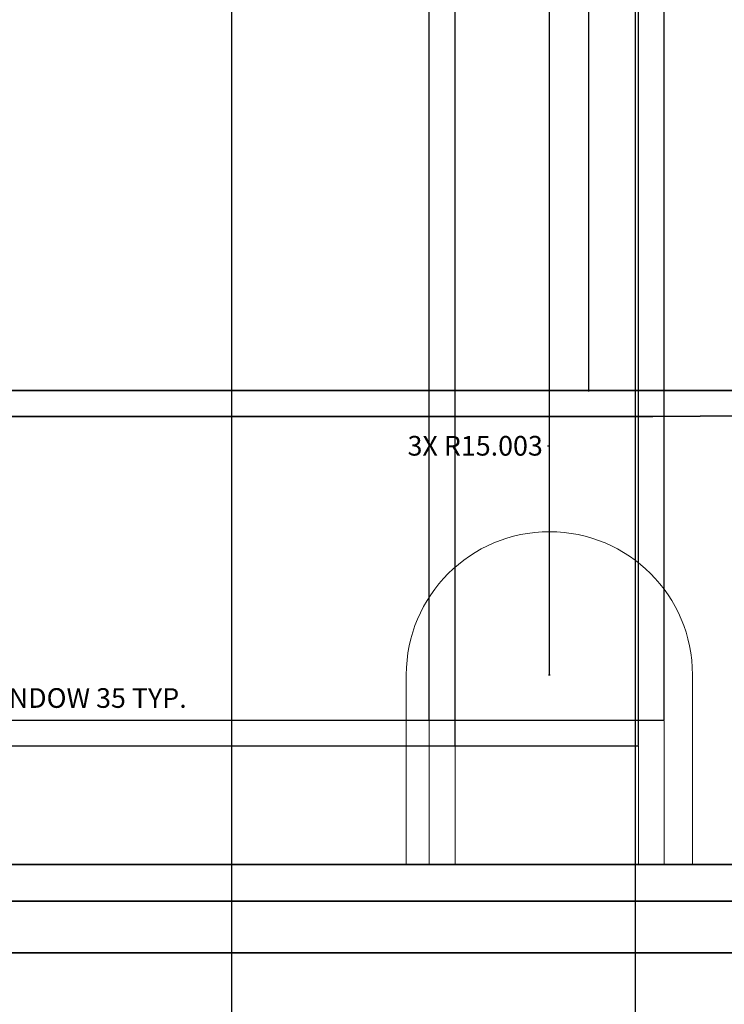
# Model space of a CAD drawing. Units: inches. Extents: x 14 to 859, y 52 to 711.
# Tile 7 of 11: x 368 to 442, y 504 to 608. Entities that reach past the tile are written whole.
import ezdxf

# ---------------------------------------------------------------- set-up
doc = ezdxf.new("R2010")
doc.units = ezdxf.units.IN
doc.header["$MEASUREMENT"] = 0
for name, color, linetype, lineweight in [('A-ANNO-DIMS', 2, 'Continuous', 18), ('A-ELEV', 7, 'Continuous', 35), ('A-GLAZ', 4, 'Continuous', 18), ('A-ROOF', 7, 'Continuous', 35)]:
    doc.layers.add(name, color=color, linetype=linetype, lineweight=lineweight)
doc.styles.get("Standard").update_dxf_attribs({"font": 'arial.ttf'})
doc.dimstyles.get("Standard").update_dxf_attribs({"dimtxt": 2.0625, "dimasz": 0.18, "dimexe": 0.18, "dimexo": 0.0625, "dimgap": 0.09, "dimtad": 0, "dimtih": 1, "dimtoh": 1, "dimdec": 4, "dimzin": 0, "dimdsep": 46, "dimlunit": 4, "dimtxsty": 'Standard', "dimcen": 0.09, "dimadec": 0, "dimazin": 0, "dimtfac": 1, "dimtdec": 4, "dimtofl": 0, "dimtmove": 0, "dimatfit": 3, "dimfxl": 1, "dimtolj": 1, "dimtzin": 0, "dimarcsym": 0})

# ---------------------------------------------------------------- blocks, each defined once
blk = doc.blocks.new('WIN-DRUM-ARCHED')
for p, q in [((329.67, 519.05), (329.67, 538.94)), ((359.68, 519.05), (359.68, 538.94))]:
    blk.add_line(p, q)
for points in [[(332.09, 519.05), (332.09, 534.15), (356.71, 534.15), (356.71, 519.05)], [(334.8, 519.05), (334.8, 531.45), (354.01, 531.45), (354.01, 519.05)]]:
    blk.add_lwpolyline(points)
blk.add_arc((344.68, 538.94), 15, 0, 180)
blk = doc.blocks.new('*D11')
at = {"layer": 'A-ANNO-DIMS', "color": 0, "lineweight": -2, "transparency": 16777216}
for p, q in [((359.74, 553.94), (365.09, 553.94)), ((364.91, 553.76), (364.91, 537.66)), ((364.91, 519.23), (364.91, 535.34)), ((359.74, 519.05), (365.09, 519.05))]:
    blk.add_line(p, q, dxfattribs=at)
at = {"layer": 'A-ANNO-DIMS', "color": 0, "transparency": 16777216}
for points in [[(364.88, 553.76), (364.94, 553.76), (364.91, 553.94)], [(364.88, 519.23), (364.94, 519.23), (364.91, 519.05)]]:
    blk.add_solid(points, dxfattribs=at)
at = {"layer": 'Defpoints', "color": 0, "transparency": 16777216}
for p in [(359.68, 553.94), (364.91, 553.94), (359.68, 519.05)]:
    blk.add_point(p, dxfattribs=at)
at = {"layer": 'A-ANNO-DIMS', "color": 0, "transparency": 16777216, "insert": (364.91, 536.5), "char_height": 2.0625, "attachment_point": 5}
blk.add_mtext('\\A1;ARCHED DRUM WINDOW 35 TYP.', dxfattribs=at)
blk = doc.blocks.new('*D13')
at = {"layer": 'A-ANNO-DIMS', "color": 0, "lineweight": -2, "transparency": 16777216}
for p, q in [((60.78, 339.73), (60.78, 709.71)), ((60.96, 709.53), (432.6, 709.53)), ((811.37, 709.53), (439.73, 709.53)), ((811.55, 339.73), (811.55, 709.71))]:
    blk.add_line(p, q, dxfattribs=at)
at = {"layer": 'A-ANNO-DIMS', "color": 0, "transparency": 16777216}
for points in [[(60.96, 709.56), (60.96, 709.5), (60.78, 709.53)], [(811.37, 709.56), (811.37, 709.5), (811.55, 709.53)]]:
    blk.add_solid(points, dxfattribs=at)
at = {"layer": 'Defpoints', "color": 0, "transparency": 16777216}
for p in [(811.55, 709.53), (60.78, 339.66), (811.55, 339.66)]:
    blk.add_point(p, dxfattribs=at)
at = {"layer": 'A-ANNO-DIMS', "color": 0, "transparency": 16777216, "insert": (436.17, 709.53), "char_height": 2.062, "attachment_point": 5}
blk.add_mtext('\\A1;750.8', dxfattribs=at)
blk = doc.blocks.new('*D16')
at = {"layer": 'A-ANNO-DIMS', "color": 0, "lineweight": -2, "transparency": 16777216}
for p, q in [((429.96, 670.76), (17.7, 670.76)), ((17.88, 670.58), (17.88, 384.41)), ((17.88, 95.97), (17.88, 382.14)), ((60.72, 95.79), (17.7, 95.79))]:
    blk.add_line(p, q, dxfattribs=at)
at = {"layer": 'A-ANNO-DIMS', "color": 0, "transparency": 16777216}
for points in [[(17.85, 670.58), (17.91, 670.58), (17.88, 670.76)], [(17.85, 95.97), (17.91, 95.97), (17.88, 95.79)]]:
    blk.add_solid(points, dxfattribs=at)
at = {"layer": 'Defpoints', "color": 0, "transparency": 16777216}
for p in [(17.88, 670.76), (430.02, 670.76), (60.78, 95.79)]:
    blk.add_point(p, dxfattribs=at)
at = {"layer": 'A-ANNO-DIMS', "color": 0, "transparency": 16777216, "insert": (17.88, 383.28), "char_height": 2.062, "attachment_point": 5}
blk.add_mtext('\\A1;575', dxfattribs=at)
blk = doc.blocks.new('*D19')
at = {"layer": 'A-ANNO-DIMS', "color": 0, "lineweight": -2, "transparency": 16777216}
for p, q in [((430.09, 670.76), (854.64, 670.76)), ((854.46, 670.58), (854.46, 538.71)), ((854.46, 404.55), (854.46, 536.42)), ((609.81, 404.37), (854.64, 404.37))]:
    blk.add_line(p, q, dxfattribs=at)
at = {"layer": 'A-ANNO-DIMS', "color": 0, "transparency": 16777216}
for points in [[(854.43, 670.58), (854.49, 670.58), (854.46, 670.76)], [(854.43, 404.55), (854.49, 404.55), (854.46, 404.37)]]:
    blk.add_solid(points, dxfattribs=at)
at = {"layer": 'Defpoints', "color": 0, "transparency": 16777216}
for p in [(430.02, 670.76), (854.46, 670.76), (609.75, 404.37)]:
    blk.add_point(p, dxfattribs=at)
at = {"layer": 'A-ANNO-DIMS', "color": 0, "transparency": 16777216, "insert": (854.46, 537.57), "char_height": 2.062, "attachment_point": 5}
blk.add_mtext('\\A1;266.4', dxfattribs=at)
blk = doc.blocks.new('*D22')
at = {"layer": 'A-ANNO-DIMS', "color": 0, "lineweight": -2, "transparency": 16777216}
for p, q in [((298.73, 341.73), (298.73, 709.71)), ((298.91, 709.53), (434.03, 709.53)), ((576.33, 709.53), (441.21, 709.53)), ((576.51, 341.73), (576.51, 709.71))]:
    blk.add_line(p, q, dxfattribs=at)
at = {"layer": 'A-ANNO-DIMS', "color": 0, "transparency": 16777216}
for points in [[(298.91, 709.56), (298.91, 709.5), (298.73, 709.53)], [(576.33, 709.56), (576.33, 709.5), (576.51, 709.53)]]:
    blk.add_solid(points, dxfattribs=at)
at = {"layer": 'Defpoints', "color": 0, "transparency": 16777216}
for p in [(576.51, 709.53), (298.73, 341.67), (576.51, 341.67)]:
    blk.add_point(p, dxfattribs=at)
at = {"layer": 'A-ANNO-DIMS', "color": 0, "transparency": 16777216, "insert": (437.62, 709.53), "char_height": 2.062, "attachment_point": 5}
blk.add_mtext('\\A1;277.8', dxfattribs=at)
blk = doc.blocks.new('*D93')
at = {"layer": 'A-ANNO-DIMS', "color": 0, "lineweight": -2, "transparency": 16777216}
for p, q in [((429.22, 654.01), (17.7, 654.01)), ((17.88, 653.83), (17.88, 612.51)), ((17.88, 568.92), (17.88, 610.23)), ((342.81, 568.74), (17.7, 568.74))]:
    blk.add_line(p, q, dxfattribs=at)
at = {"layer": 'A-ANNO-DIMS', "color": 0, "transparency": 16777216}
for points in [[(17.85, 653.83), (17.91, 653.83), (17.88, 654.01)], [(17.85, 568.92), (17.91, 568.92), (17.88, 568.74)]]:
    blk.add_solid(points, dxfattribs=at)
at = {"layer": 'Defpoints', "color": 0, "transparency": 16777216}
for p in [(17.88, 654.01), (429.29, 654.01), (342.87, 568.74)]:
    blk.add_point(p, dxfattribs=at)
at = {"layer": 'A-ANNO-DIMS', "color": 0, "transparency": 16777216, "insert": (17.88, 611.37), "char_height": 2.062, "attachment_point": 5}
blk.add_mtext('\\A1;85.27', dxfattribs=at)
blk = doc.blocks.new('*D97')
at = {"layer": 'A-ANNO-DIMS', "color": 0, "lineweight": -2, "transparency": 16777216}
for p, q in [((366.51, 447.01), (366.51, 709.71)), ((366.69, 709.53), (396.2, 709.53)), ((432.88, 709.53), (403.37, 709.53)), ((433.06, 447.01), (433.06, 709.71))]:
    blk.add_line(p, q, dxfattribs=at)
at = {"layer": 'A-ANNO-DIMS', "color": 0, "transparency": 16777216}
for points in [[(366.69, 709.56), (366.69, 709.5), (366.51, 709.53)], [(432.88, 709.56), (432.88, 709.5), (433.06, 709.53)]]:
    blk.add_solid(points, dxfattribs=at)
at = {"layer": 'Defpoints', "color": 0, "transparency": 16777216}
for p in [(433.06, 709.53), (366.51, 446.95), (433.06, 446.95)]:
    blk.add_point(p, dxfattribs=at)
at = {"layer": 'A-ANNO-DIMS', "color": 0, "transparency": 16777216, "insert": (399.78, 709.53), "char_height": 2.062, "attachment_point": 5}
blk.add_mtext('\\A1;66.55', dxfattribs=at)
blk = doc.blocks.new('*D98')
at = {"layer": 'A-ANNO-DIMS', "color": 0, "lineweight": -2, "transparency": 16777216}
for p, q in [((433.06, 447.01), (433.06, 709.71)), ((433.24, 709.53), (465.59, 709.53)), ((505.07, 709.53), (472.72, 709.53)), ((505.25, 447.01), (505.25, 709.71))]:
    blk.add_line(p, q, dxfattribs=at)
at = {"layer": 'A-ANNO-DIMS', "color": 0, "transparency": 16777216}
for points in [[(433.24, 709.56), (433.24, 709.5), (433.06, 709.53)], [(505.07, 709.56), (505.07, 709.5), (505.25, 709.53)]]:
    blk.add_solid(points, dxfattribs=at)
at = {"layer": 'Defpoints', "color": 0, "transparency": 16777216}
for p in [(505.25, 709.53), (433.06, 446.95), (505.25, 446.95)]:
    blk.add_point(p, dxfattribs=at)
at = {"layer": 'A-ANNO-DIMS', "color": 0, "transparency": 16777216, "insert": (469.15, 709.53), "char_height": 2.062, "attachment_point": 5}
blk.add_mtext('\\A1;72.19', dxfattribs=at)
blk = doc.blocks.new('*D105')
at = {"layer": 'A-ANNO-DIMS', "color": 0, "lineweight": -2, "transparency": 16777216}
for p, q in [((306.86, 560.74), (306.86, 709.71)), ((307.04, 709.53), (424.56, 709.53)), ((549.26, 709.53), (431.74, 709.53)), ((549.44, 560.74), (549.44, 709.71))]:
    blk.add_line(p, q, dxfattribs=at)
at = {"layer": 'A-ANNO-DIMS', "color": 0, "transparency": 16777216}
for points in [[(307.04, 709.56), (307.04, 709.5), (306.86, 709.53)], [(549.26, 709.56), (549.26, 709.5), (549.44, 709.53)]]:
    blk.add_solid(points, dxfattribs=at)
at = {"layer": 'Defpoints', "color": 0, "transparency": 16777216}
for p in [(549.44, 709.53), (306.86, 560.68), (549.44, 560.68)]:
    blk.add_point(p, dxfattribs=at)
at = {"layer": 'A-ANNO-DIMS', "color": 0, "transparency": 16777216, "insert": (428.15, 709.53), "char_height": 2.062, "attachment_point": 5}
blk.add_mtext('\\A1;242.6', dxfattribs=at)
blk = doc.blocks.new('*D111')
at = {"layer": 'A-ANNO-DIMS', "color": 0, "lineweight": -2, "transparency": 16777216}
for p, q in [((344.68, 539), (344.68, 709.71)), ((344.86, 709.53), (380.79, 709.53)), ((423.84, 709.53), (387.91, 709.53)), ((424.02, 539), (424.02, 709.71))]:
    blk.add_line(p, q, dxfattribs=at)
at = {"layer": 'A-ANNO-DIMS', "color": 0, "transparency": 16777216}
for points in [[(344.86, 709.56), (344.86, 709.5), (344.68, 709.53)], [(423.84, 709.56), (423.84, 709.5), (424.02, 709.53)]]:
    blk.add_solid(points, dxfattribs=at)
at = {"layer": 'Defpoints', "color": 0, "transparency": 16777216}
for p in [(424.02, 709.53), (344.68, 538.94), (424.02, 538.94)]:
    blk.add_point(p, dxfattribs=at)
at = {"layer": 'A-ANNO-DIMS', "color": 0, "transparency": 16777216, "insert": (384.35, 709.53), "char_height": 2.062, "attachment_point": 5}
blk.add_mtext('\\A1;79.34', dxfattribs=at)
blk = doc.blocks.new('*D112')
at = {"layer": 'A-ANNO-DIMS', "color": 0, "lineweight": -2, "transparency": 16777216}
for p, q in [((424.02, 539), (424.02, 709.71)), ((424.2, 709.53), (462.95, 709.53)), ((508.45, 709.53), (469.7, 709.53)), ((508.63, 539), (508.63, 709.71))]:
    blk.add_line(p, q, dxfattribs=at)
at = {"layer": 'A-ANNO-DIMS', "color": 0, "transparency": 16777216}
for points in [[(424.2, 709.56), (424.2, 709.5), (424.02, 709.53)], [(508.45, 709.56), (508.45, 709.5), (508.63, 709.53)]]:
    blk.add_solid(points, dxfattribs=at)
at = {"layer": 'Defpoints', "color": 0, "transparency": 16777216}
for p in [(508.63, 709.53), (424.02, 538.94), (508.63, 538.94)]:
    blk.add_point(p, dxfattribs=at)
at = {"layer": 'A-ANNO-DIMS', "color": 0, "transparency": 16777216, "insert": (466.32, 709.53), "char_height": 2.062, "attachment_point": 5}
blk.add_mtext('\\A1;84.61', dxfattribs=at)
blk = doc.blocks.new('*D114')
at = {"layer": 'A-ANNO-DIMS', "color": 0, "lineweight": -2, "transparency": 16777216}
for p, q in [((411.43, 534.21), (411.43, 709.71)), ((411.61, 709.53), (420.17, 709.53)), ((435.87, 709.53), (427.32, 709.53)), ((436.05, 534.21), (436.05, 709.71))]:
    blk.add_line(p, q, dxfattribs=at)
at = {"layer": 'A-ANNO-DIMS', "color": 0, "transparency": 16777216}
for points in [[(411.61, 709.56), (411.61, 709.5), (411.43, 709.53)], [(435.87, 709.56), (435.87, 709.5), (436.05, 709.53)]]:
    blk.add_solid(points, dxfattribs=at)
at = {"layer": 'Defpoints', "color": 0, "transparency": 16777216}
for p in [(436.05, 709.53), (411.43, 534.15), (436.05, 534.15)]:
    blk.add_point(p, dxfattribs=at)
at = {"layer": 'A-ANNO-DIMS', "color": 0, "transparency": 16777216, "insert": (423.74, 709.53), "char_height": 2.062, "attachment_point": 5}
blk.add_mtext('\\A1;24.62', dxfattribs=at)
blk = doc.blocks.new('*D115')
at = {"layer": 'A-ANNO-DIMS', "color": 0, "lineweight": -2, "transparency": 16777216}
for p, q in [((414.14, 531.51), (414.14, 709.71)), ((414.32, 709.53), (420.47, 709.53)), ((433.17, 709.53), (427.02, 709.53)), ((433.35, 531.51), (433.35, 709.71))]:
    blk.add_line(p, q, dxfattribs=at)
at = {"layer": 'A-ANNO-DIMS', "color": 0, "transparency": 16777216}
for points in [[(414.32, 709.56), (414.32, 709.5), (414.14, 709.53)], [(433.17, 709.56), (433.17, 709.5), (433.35, 709.53)]]:
    blk.add_solid(points, dxfattribs=at)
at = {"layer": 'Defpoints', "color": 0, "transparency": 16777216}
for p in [(433.35, 709.53), (414.14, 531.45), (433.35, 531.45)]:
    blk.add_point(p, dxfattribs=at)
at = {"layer": 'A-ANNO-DIMS', "color": 0, "transparency": 16777216, "insert": (423.74, 709.53), "char_height": 2.062, "attachment_point": 5}
blk.add_mtext('\\A1;19.21', dxfattribs=at)
blk = doc.blocks.new('*D116')
at = {"layer": 'A-ANNO-DIMS', "color": 0, "lineweight": -2, "transparency": 16777216}
for p, q in [((435.99, 534.15), (17.7, 534.15)), ((17.88, 533.97), (17.88, 527.74)), ((17.88, 519.23), (17.88, 525.46)), ((435.99, 519.05), (17.7, 519.05))]:
    blk.add_line(p, q, dxfattribs=at)
at = {"layer": 'A-ANNO-DIMS', "color": 0, "transparency": 16777216}
for points in [[(17.85, 533.97), (17.91, 533.97), (17.88, 534.15)], [(17.85, 519.23), (17.91, 519.23), (17.88, 519.05)]]:
    blk.add_solid(points, dxfattribs=at)
at = {"layer": 'Defpoints', "color": 0, "transparency": 16777216}
for p in [(17.88, 534.15), (436.05, 534.15), (436.05, 519.05)]:
    blk.add_point(p, dxfattribs=at)
at = {"layer": 'A-ANNO-DIMS', "color": 0, "transparency": 16777216, "insert": (17.88, 526.6), "char_height": 2.062, "attachment_point": 5}
blk.add_mtext('\\A1;15.1', dxfattribs=at)
blk = doc.blocks.new('*D117')
at = {"layer": 'A-ANNO-DIMS', "color": 0, "lineweight": -2, "transparency": 16777216}
for p, q in [((433.29, 531.45), (17.7, 531.45)), ((17.88, 531.27), (17.88, 526.39)), ((17.88, 519.23), (17.88, 524.11)), ((433.29, 519.05), (17.7, 519.05))]:
    blk.add_line(p, q, dxfattribs=at)
at = {"layer": 'A-ANNO-DIMS', "color": 0, "transparency": 16777216}
for points in [[(17.85, 531.27), (17.91, 531.27), (17.88, 531.45)], [(17.85, 519.23), (17.91, 519.23), (17.88, 519.05)]]:
    blk.add_solid(points, dxfattribs=at)
at = {"layer": 'Defpoints', "color": 0, "transparency": 16777216}
for p in [(17.88, 531.45), (433.35, 531.45), (433.35, 519.05)]:
    blk.add_point(p, dxfattribs=at)
at = {"layer": 'A-ANNO-DIMS', "color": 0, "transparency": 16777216, "insert": (17.88, 525.25), "char_height": 2.062, "attachment_point": 5}
blk.add_mtext('\\A1;12.395', dxfattribs=at)
blk = doc.blocks.new('*D118')
at = {"layer": 'A-ANNO-DIMS', "color": 0, "lineweight": -2, "transparency": 16777216}
for p, q in [((306.86, 560.74), (306.86, 709.71)), ((307.04, 709.53), (364.03, 709.53)), ((427.97, 709.53), (370.98, 709.53)), ((428.15, 568.8), (428.15, 709.71))]:
    blk.add_line(p, q, dxfattribs=at)
at = {"layer": 'A-ANNO-DIMS', "color": 0, "transparency": 16777216}
for points in [[(307.04, 709.56), (307.04, 709.5), (306.86, 709.53)], [(427.97, 709.56), (427.97, 709.5), (428.15, 709.53)]]:
    blk.add_solid(points, dxfattribs=at)
at = {"layer": 'Defpoints', "color": 0, "transparency": 16777216}
for p in [(428.15, 709.53), (428.15, 568.74), (306.86, 560.68)]:
    blk.add_point(p, dxfattribs=at)
at = {"layer": 'A-ANNO-DIMS', "color": 0, "transparency": 16777216, "insert": (367.51, 709.53), "char_height": 2.062, "attachment_point": 5}
blk.add_mtext('\\A1;121.3', dxfattribs=at)
blk = doc.blocks.new('*D120')
at = {"layer": 'A-ANNO-DIMS', "color": 0, "lineweight": -2, "transparency": 16777216}
for p, q in [((324.18, 404.43), (324.18, 709.71)), ((324.36, 709.53), (353.87, 709.53)), ((390.55, 709.53), (361.04, 709.53)), ((390.73, 404.43), (390.73, 709.71))]:
    blk.add_line(p, q, dxfattribs=at)
at = {"layer": 'A-ANNO-DIMS', "color": 0, "transparency": 16777216}
for points in [[(324.36, 709.56), (324.36, 709.5), (324.18, 709.53)], [(390.55, 709.56), (390.55, 709.5), (390.73, 709.53)]]:
    blk.add_solid(points, dxfattribs=at)
at = {"layer": 'Defpoints', "color": 0, "transparency": 16777216}
for p in [(390.73, 709.53), (324.18, 404.37), (390.73, 404.37)]:
    blk.add_point(p, dxfattribs=at)
at = {"layer": 'A-ANNO-DIMS', "color": 0, "transparency": 16777216, "insert": (357.45, 709.53), "char_height": 2.062, "attachment_point": 5}
blk.add_mtext('\\A1;66.55', dxfattribs=at)
blk = doc.blocks.new('*D121')
at = {"layer": 'A-ANNO-DIMS', "color": 0, "lineweight": -2, "transparency": 16777216}
for p, q in [((390.73, 404.43), (390.73, 709.71)), ((390.91, 709.53), (416.86, 709.53)), ((448.36, 709.53), (422.4, 709.53)), ((448.54, 404.43), (448.54, 709.71))]:
    blk.add_line(p, q, dxfattribs=at)
at = {"layer": 'A-ANNO-DIMS', "color": 0, "transparency": 16777216}
for points in [[(390.91, 709.56), (390.91, 709.5), (390.73, 709.53)], [(448.36, 709.56), (448.36, 709.5), (448.54, 709.53)]]:
    blk.add_solid(points, dxfattribs=at)
at = {"layer": 'Defpoints', "color": 0, "transparency": 16777216}
for p in [(448.54, 709.53), (390.73, 404.37), (448.54, 404.37)]:
    blk.add_point(p, dxfattribs=at)
at = {"layer": 'A-ANNO-DIMS', "color": 0, "transparency": 16777216, "insert": (419.63, 709.53), "char_height": 2.062, "attachment_point": 5}
blk.add_mtext('\\A1;57.8', dxfattribs=at)
blk = doc.blocks.new('*D130')
at = {"layer": 'A-ANNO-DIMS', "color": 0, "lineweight": -2, "transparency": 16777216}
for p, q in [((541.65, 644.46), (499.24, 616.16)), ((541.83, 644.46), (541.65, 644.46)), ((428.06, 568.74), (428.24, 568.74)), ((428.15, 568.65), (428.15, 568.83))]:
    blk.add_line(p, q, dxfattribs=at)
at = {"layer": 'A-ANNO-DIMS', "color": 0, "transparency": 16777216}
blk.add_solid([(499.22, 616.19), (499.26, 616.14), (499.09, 616.06)], dxfattribs=at)
at = {"layer": 'Defpoints', "color": 0, "transparency": 16777216}
for p in [(499.09, 616.06), (428.15, 568.74)]:
    blk.add_point(p, dxfattribs=at)
at = {"layer": 'A-ANNO-DIMS', "color": 0, "transparency": 16777216, "insert": (546.39, 644.46), "char_height": 2.062, "attachment_point": 5}
blk.add_mtext('\\A1;R85.28', dxfattribs=at)
blk = doc.blocks.new('*D132')
at = {"layer": 'A-ANNO-DIMS', "color": 0, "lineweight": -2, "transparency": 16777216}
for p, q in [((423.81, 562.95), (423.99, 562.95)), ((423.99, 562.95), (424, 554.12)), ((424.02, 538.85), (424.02, 539.03)), ((423.93, 538.94), (424.11, 538.94))]:
    blk.add_line(p, q, dxfattribs=at)
at = {"layer": 'A-ANNO-DIMS', "color": 0, "transparency": 16777216}
blk.add_solid([(424.03, 554.12), (423.97, 554.12), (424, 553.94)], dxfattribs=at)
at = {"layer": 'Defpoints', "color": 0, "transparency": 16777216}
for p in [(424, 553.94), (424.02, 538.94)]:
    blk.add_point(p, dxfattribs=at)
at = {"layer": 'A-ANNO-DIMS', "color": 0, "transparency": 16777216, "insert": (416.24, 562.95), "char_height": 2.0625, "attachment_point": 5}
blk.add_mtext('\\A1;3X R15.003', dxfattribs=at)

msp = doc.modelspace()

# ---------------------------------------------------------------- linework, layer by layer
at = {"layer": 'A-ELEV'}
for p, q in [((342.8739, 568.7358), (434.8803, 568.7358)), ((434.8803, 568.7358), (513.4296, 568.7358)), ((343.0726, 566.0314), (434.8803, 566.0314)), ((434.8803, 566.0314), (513.3994, 566.4671)), ((264.6274, 519.0512), (555.2103, 519.0512)), ((276.5038, 515.1991), (537.6873, 515.1991)), ((276.5038, 509.7903), (537.6873, 509.7903))]:
    msp.add_line(p, q, dxfattribs=at)
at = {"layer": 'A-ROOF'}
msp.add_arc((428.1517, 568.7358), 85.2778, 358.475544, 180, dxfattribs=at)

# ---------------------------------------------------------------- block references
at = {"layer": 'A-GLAZ'}
msp.add_blockref('WIN-DRUM-ARCHED', (79.3415, 0), dxfattribs=at)

# ---------------------------------------------------------------- dimensions: what is measured, and where the dimension line sits
at = {"layer": 'A-ANNO-DIMS'}
for base, p1, p2, override, picture, middle in [((811.5534, 709.5262), (60.7804, 339.6626), (811.5534, 339.6626), {"dimdec": 1, "dimlfac": 1, "dimrnd": 0, "dimzin": 0, "dimdsep": 46, "dimlunit": 2}, '*D13', (436.1669, 709.5262)), ((576.5058, 709.5262), (298.7295, 341.6716), (576.5058, 341.6716), {"dimdec": 1, "dimlfac": 1, "dimrnd": 0, "dimzin": 0, "dimdsep": 46, "dimlunit": 2}, '*D22', (437.6176, 709.5262)), ((549.4429, 709.5262), (306.8606, 560.6808), (549.4429, 560.6808), {"dimdec": 1, "dimlfac": 1, "dimrnd": 0, "dimzin": 0, "dimdsep": 46, "dimlunit": 2}, '*D105', (428.1517, 709.5262)), ((428.1517, 709.5262), (306.8606, 560.6808), (428.1517, 568.7358), {"dimdec": 1, "dimlfac": 1, "dimrnd": 0, "dimzin": 0, "dimdsep": 46, "dimlunit": 2}, '*D118', (367.5062, 709.5262)), ((390.7307, 709.5262), (324.1777, 404.3712), (390.7307, 404.3712), {"dimdec": 2, "dimlfac": 1, "dimrnd": 0, "dimzin": 0, "dimdsep": 46, "dimlunit": 2}, '*D120', (357.4542, 709.5262)), ((424.0193, 709.5262), (344.6778, 538.9419), (424.0193, 538.9419), {"dimdec": 2, "dimlfac": 1, "dimrnd": 0, "dimzin": 0, "dimdsep": 46, "dimlunit": 2}, '*D111', (384.3486, 709.5262)), ((433.06, 709.5262), (366.507, 446.9501), (433.06, 446.9501), {"dimdec": 2, "dimlfac": 1, "dimrnd": 0, "dimzin": 0, "dimdsep": 46, "dimlunit": 2}, '*D97', (399.7835, 709.5262)), ((448.5359, 709.5262), (390.7307, 404.3712), (448.5359, 404.3712), {"dimdec": 1, "dimlfac": 1, "dimrnd": 0, "dimzin": 0, "dimdsep": 46, "dimlunit": 2}, '*D121', (419.6333, 709.5262)), ((436.0547, 709.5262), (411.435, 534.1509), (436.0547, 534.1509), {"dimdec": 2, "dimlfac": 1, "dimrnd": 0, "dimzin": 0, "dimdsep": 46, "dimlunit": 2}, '*D114', (423.7449, 709.5262)), ((433.3504, 709.5262), (414.1394, 531.4465), (433.3504, 531.4465), {"dimdec": 2, "dimlfac": 1, "dimrnd": 0, "dimzin": 0, "dimdsep": 46, "dimlunit": 2}, '*D115', (423.7449, 709.5262)), ((508.63, 709.5262), (424.0193, 538.9419), (508.63, 538.9419), {"dimdec": 2, "dimlfac": 1, "dimrnd": 0, "dimzin": 0, "dimdsep": 46, "dimlunit": 2}, '*D112', (466.3247, 709.5262)), ((505.2493, 709.5262), (433.06, 446.9501), (505.2493, 446.9501), {"dimdec": 2, "dimlfac": 1, "dimrnd": 0, "dimzin": 0, "dimdsep": 46, "dimlunit": 2}, '*D98', (469.1547, 709.5262))]:
    dim = msp.add_linear_dim(base=base, p1=p1, p2=p2, dimstyle='Standard', override=override, dxfattribs=at)
    dim.commit()
    dim.dimension.update_dxf_attribs({"geometry": picture, "text_midpoint": middle})
for base, p1, p2, override, picture, middle in [((17.8785, 670.7637), (60.7804, 95.7876), (430.0228, 670.7637), {"dimdec": 0, "dimlfac": 1, "dimrnd": 0, "dimzin": 0, "dimdsep": 46, "dimlunit": 2}, '*D16', (17.8785, 383.2756)), ((854.4554, 670.7637), (609.7501, 404.3712), (430.0228, 670.7637), {"dimdec": 1, "dimlfac": 1, "dimrnd": 0, "dimzin": 0, "dimdsep": 46, "dimlunit": 2}, '*D19', (854.4554, 537.5675)), ((17.8785, 654.0061), (342.8739, 568.7358), (429.2862, 654.0061), {"dimdec": 2, "dimlfac": 1, "dimrnd": 0, "dimzin": 0, "dimdsep": 46, "dimlunit": 2}, '*D93', (17.8785, 611.371)), ((17.8785, 534.1509), (436.0547, 519.0512), (436.0547, 534.1509), {"dimdec": 1, "dimlfac": 1, "dimrnd": 0, "dimzin": 0, "dimdsep": 46, "dimlunit": 2}, '*D116', (17.8785, 526.601)), ((17.8785, 531.4465), (433.3504, 519.0512), (433.3504, 531.4465), {"dimdec": 3, "dimlfac": 1, "dimrnd": 0, "dimzin": 0, "dimdsep": 46, "dimlunit": 2}, '*D117', (17.8785, 525.2488))]:
    dim = msp.add_linear_dim(base=base, p1=p1, p2=p2, angle=90, dimstyle='Standard', override=override, dxfattribs=at)
    dim.commit()
    dim.dimension.update_dxf_attribs({"geometry": picture, "text_midpoint": middle})
dim = msp.add_radius_dim(center=(428.1517, 568.7358), mpoint=(499.0902, 616.0649), dimstyle='Standard', override={"dimdec": 2, "dimlfac": 1, "dimrnd": 0, "dimzin": 0, "dimdsep": 46, "dimlunit": 2}, dxfattribs=at)
dim.commit()
dim.dimension.update_dxf_attribs({"geometry": '*D130', "text_midpoint": (546.3923, 644.4623), "dimtype": 164})
dim = msp.add_radius_dim(center=(424.0193, 538.9419), mpoint=(423.9999, 553.9447), text='3X <>', dimstyle='Standard', override={"dimdec": 3, "dimlfac": 1, "dimrnd": 0, "dimzin": 0, "dimdsep": 46, "dimlunit": 2}, dxfattribs=at)
dim.commit()
dim.dimension.update_dxf_attribs({"geometry": '*D132', "text_midpoint": (416.2351, 562.9464), "dimtype": 164})
dim = msp.add_linear_dim(base=(364.9147, 553.9447), p1=(359.6807, 519.0512), p2=(359.6807, 553.9447), angle=90, text='ARCHED DRUM WINDOW <> TYP.', dimstyle='Standard', override={"dimdec": 0, "dimlfac": 1, "dimrnd": 0, "dimzin": 0, "dimdsep": 46, "dimlunit": 2}, dxfattribs=at)
dim.commit()
dim.dimension.update_dxf_attribs({"geometry": '*D11', "text_midpoint": (364.9147, 536.498)})

doc.saveas('drawing.dxf')
